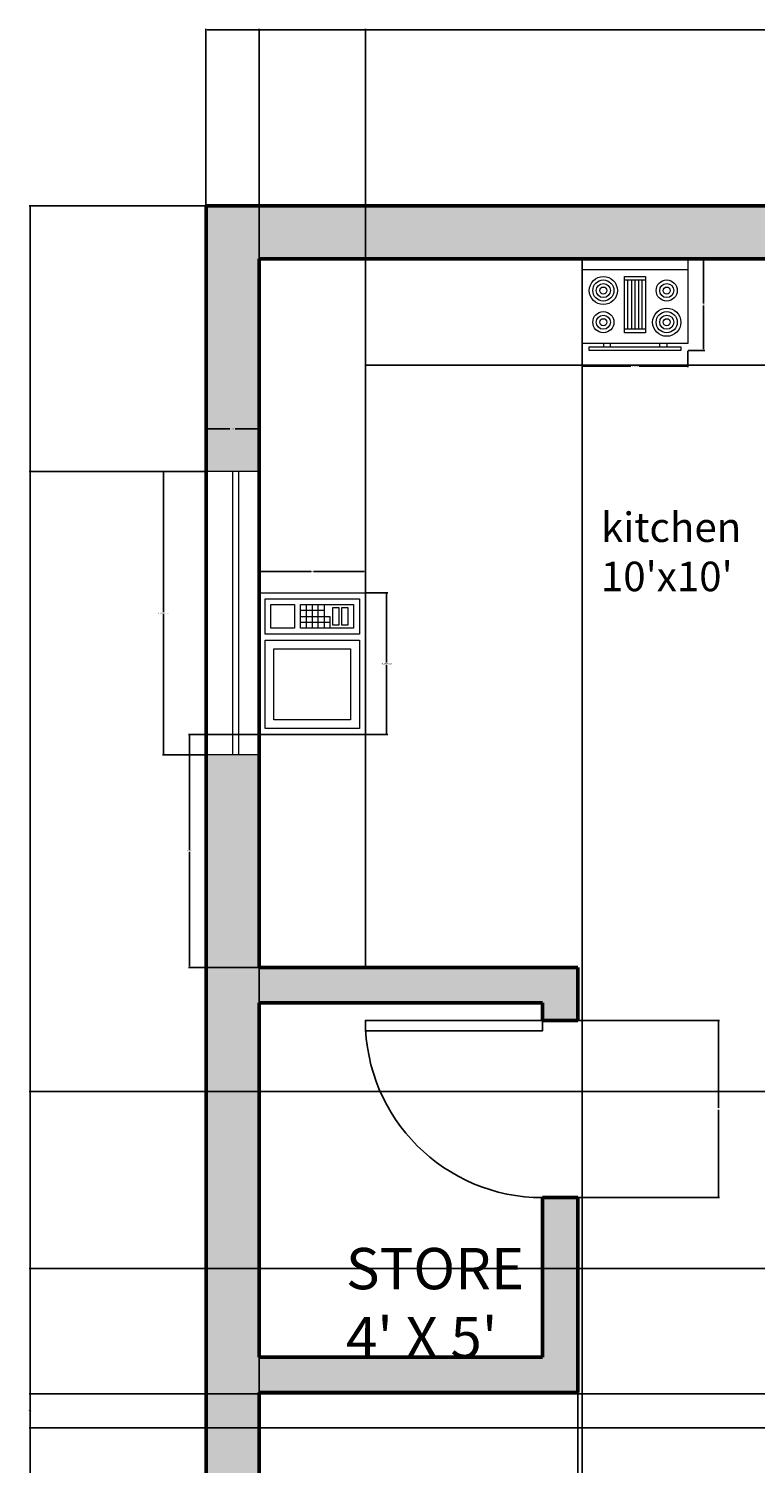
# Model space of a CAD drawing. Units: inches. Extents: x 1489 to 1813, y 1703 to 2293.
# Tile 3 of 4: x 1489 to 1612, y 2050 to 2293. Entities that reach past the tile are written whole.
import ezdxf

# ---------------------------------------------------------------- set-up
doc = ezdxf.new("R2010")
doc.units = ezdxf.units.IN
doc.header["$LTSCALE"] = 0.4
doc.linetypes.add('HIDDEN', pattern=[9.525, 6.35, -3.175])
for name, color, linetype, lineweight in [('A-ANNO-DIMS', 2, 'Continuous', 18), ('A-AREA-IDEN', 7, 'Continuous', 18), ('A-DOOR', 4, 'Continuous', 25), ('A-EQPM', 9, 'Continuous', 18), ('A-FLOR-CASE', 8, 'Continuous', 25), ('A-GLAZ', 4, 'Continuous', 18), ('A-WALL', 7, 'Continuous', 50)]:
    doc.layers.add(name, color=color, linetype=linetype, lineweight=lineweight)
doc.layers.add('A-WALL-PATT', color=18, linetype='HIDDEN', lineweight=13, true_color=0x000000)
doc.styles.get("Standard").update_dxf_attribs({"font": 'arial.ttf'})
doc.dimstyles.get("Standard").update_dxf_attribs({"dimtxt": 0.18, "dimasz": 0.18, "dimexe": 0.18, "dimexo": 0.0625, "dimgap": 0.09, "dimtad": 0, "dimtih": 1, "dimtoh": 1, "dimdec": 4, "dimzin": 0, "dimdsep": 46, "dimtxsty": 'Standard', "dimcen": 0.09, "dimadec": 0, "dimazin": 0, "dimtfac": 1, "dimtdec": 4, "dimtofl": 0, "dimtmove": 0, "dimatfit": 3, "dimfxl": 1, "dimtolj": 1, "dimtzin": 0, "dimarcsym": 0})

# ---------------------------------------------------------------- blocks, each defined once
blk = doc.blocks.new('*U3')
for p, q in [((0, 0), (0, -6)), ((30, 0), (30, -6))]:
    blk.add_line(p, q)
blk.add_lwpolyline([(0, 0), (0, 30), (1.75, 30), (1.75, 0)], close=True)
blk.add_arc((0, 0), 30, 0, 90)
blk = doc.blocks.new('Range-Oven - 30 in top')
for p, q in [((0, -3), (30, -3)), ((12, -6), (18, -6)), ((13, -20), (13, -6)), ((14, -6), (14, -20)), ((15, -20), (15, -6)), ((16, -6), (16, -20)), ((17, -20), (17, -6)), ((18, -20), (12, -20)), ((6, -24), (6, -25)), ((8, -25), (8, -24)), ((22, -25), (22, -24)), ((24, -24), (24, -25))]:
    blk.add_line(p, q)
for points in [[(0, -24), (0, 0), (30, 0), (30, -24)], [(12, -21), (12, -5), (18, -5), (18, -21)], [(2, -26), (2, -25), (28, -25), (28, -26)]]:
    blk.add_lwpolyline(points, close=True)
for centre, radius in [((6, -9), 4), ((6, -9), 3), ((6, -9), 2), ((6, -9), 1), ((24, -9), 3), ((24, -9), 2), ((24, -9), 1), ((6, -18), 3), ((6, -18), 2), ((24, -18), 4), ((24, -18), 3), ((24, -18), 2), ((6, -18), 1), ((24, -18), 1)]:
    blk.add_circle(centre, radius)
blk = doc.blocks.new('Microwave')
for p, q in [((18, 10), (22, 10)), ((19, 7), (19, 11)), ((20, 11), (20, 7)), ((21, 7), (21, 11)), ((22, 9), (18, 9)), ((18, 8), (22, 8)), ((22, 7), (18, 7)), ((20, 6), (18, 6)), ((19, 6), (19, 7)), ((20, 7), (20, 6))]:
    blk.add_line(p, q)
for points in [[(0, 0), (0, 18), (24, 18), (24, 0)], [(1, 1), (1, 17), (16, 17), (16, 1)], [(2.5, 2.5), (2.5, 15.5), (14.5, 15.5), (14.5, 2.5)], [(17, 1), (17, 17), (23, 17), (23, 1)], [(18, 12), (18, 16), (22, 16), (22, 12)], [(18, 2), (18, 11), (22, 11), (22, 2)], [(18.5, 4.5), (18.5, 5.5), (21.5, 5.5), (21.5, 4.5)], [(18.5, 3), (18.5, 4), (21.5, 4), (21.5, 3)]]:
    blk.add_lwpolyline(points, close=True)
blk = doc.blocks.new('WIN-48IN')
for p, q in [((9, 48), (0, 48)), ((4.5, 48), (4.5, 0)), ((5.5, 48), (5.5, 0)), ((9, 0), (0, 0))]:
    blk.add_line(p, q)
blk = doc.blocks.new('*D14')
at = {"layer": 'A-ANNO-DIMS', "color": 0, "lineweight": -2, "ltscale": 0.4, "transparency": 16777216}
for p, q in [((1518.92, 2218.17), (1511.6, 2218.17)), ((1511.78, 2217.99), (1511.78, 2194.35)), ((1511.78, 2170.35), (1511.78, 2193.99)), ((1518.92, 2170.17), (1511.6, 2170.17))]:
    blk.add_line(p, q, dxfattribs=at)
at = {"layer": 'A-ANNO-DIMS', "color": 0, "ltscale": 0.4, "transparency": 16777216}
for points in [[(1511.75, 2217.99), (1511.81, 2217.99), (1511.78, 2218.17)], [(1511.75, 2170.35), (1511.81, 2170.35), (1511.78, 2170.17)]]:
    blk.add_solid(points, dxfattribs=at)
at = {"layer": 'Defpoints', "color": 0, "ltscale": 0.4, "transparency": 16777216}
for p in [(1511.78, 2218.17), (1518.98, 2218.17), (1518.98, 2170.17)]:
    blk.add_point(p, dxfattribs=at)
at = {"layer": 'A-ANNO-DIMS', "color": 0, "ltscale": 0.4, "transparency": 16777216, "insert": (1511.78, 2194.17), "char_height": 0.18, "attachment_point": 5}
blk.add_mtext('\\A1;WINDOW 48 TYP.', dxfattribs=at)
blk = doc.blocks.new('*D15')
at = {"layer": 'A-ANNO-DIMS', "color": 0, "lineweight": -2, "ltscale": 0.4, "transparency": 16777216}
for p, q in [((1518.98, 2218.23), (1518.98, 2225.55)), ((1519.16, 2225.37), (1523.03, 2225.37)), ((1527.8, 2225.37), (1523.94, 2225.37)), ((1527.98, 2218.23), (1527.98, 2225.55))]:
    blk.add_line(p, q, dxfattribs=at)
at = {"layer": 'A-ANNO-DIMS', "color": 0, "ltscale": 0.4, "transparency": 16777216}
for points in [[(1519.16, 2225.4), (1519.16, 2225.34), (1518.98, 2225.37)], [(1527.8, 2225.4), (1527.8, 2225.34), (1527.98, 2225.37)]]:
    blk.add_solid(points, dxfattribs=at)
at = {"layer": 'Defpoints', "color": 0, "ltscale": 0.4, "transparency": 16777216}
for p in [(1527.98, 2225.37), (1518.98, 2218.17), (1527.98, 2218.17)]:
    blk.add_point(p, dxfattribs=at)
at = {"layer": 'A-ANNO-DIMS', "color": 0, "ltscale": 0.4, "transparency": 16777216, "insert": (1523.48, 2225.37), "char_height": 0.18, "attachment_point": 5}
blk.add_mtext('\\A1;9 TYP.', dxfattribs=at)
blk = doc.blocks.new('*D22')
at = {"layer": 'A-ANNO-DIMS', "color": 0, "lineweight": -2, "ltscale": 0.4, "transparency": 16777216}
for p, q in [((1582.71, 2238.6), (1582.71, 2235.8)), ((1600.6, 2238.6), (1600.6, 2235.8)), ((1582.89, 2235.98), (1590.96, 2235.98)), ((1600.42, 2235.98), (1592.35, 2235.98))]:
    blk.add_line(p, q, dxfattribs=at)
at = {"layer": 'A-ANNO-DIMS', "color": 0, "ltscale": 0.4, "transparency": 16777216}
for points in [[(1582.89, 2236.01), (1582.89, 2235.95), (1582.71, 2235.98)], [(1600.42, 2236.01), (1600.42, 2235.95), (1600.6, 2235.98)]]:
    blk.add_solid(points, dxfattribs=at)
at = {"layer": 'Defpoints', "color": 0, "ltscale": 0.4, "transparency": 16777216}
for p in [(1582.71, 2238.67), (1600.6, 2238.67), (1600.6, 2235.98)]:
    blk.add_point(p, dxfattribs=at)
at = {"layer": 'A-ANNO-DIMS', "color": 0, "ltscale": 0.4, "transparency": 16777216, "insert": (1591.66, 2235.98), "char_height": 0.18, "attachment_point": 5}
blk.add_mtext('\\A1;RANGE 18', dxfattribs=at)
blk = doc.blocks.new('*D23')
at = {"layer": 'A-ANNO-DIMS', "color": 0, "lineweight": -2, "ltscale": 0.4, "transparency": 16777216}
for p, q in [((1600.66, 2254.17), (1603.46, 2254.17)), ((1603.28, 2253.99), (1603.28, 2246.6)), ((1603.28, 2238.85), (1603.28, 2246.24)), ((1600.66, 2238.67), (1603.46, 2238.67))]:
    blk.add_line(p, q, dxfattribs=at)
at = {"layer": 'A-ANNO-DIMS', "color": 0, "ltscale": 0.4, "transparency": 16777216}
for points in [[(1603.25, 2253.99), (1603.31, 2253.99), (1603.28, 2254.17)], [(1603.25, 2238.85), (1603.31, 2238.85), (1603.28, 2238.67)]]:
    blk.add_solid(points, dxfattribs=at)
at = {"layer": 'Defpoints', "color": 0, "ltscale": 0.4, "transparency": 16777216}
for p in [(1600.6, 2254.17), (1603.28, 2254.17), (1600.6, 2238.67)]:
    blk.add_point(p, dxfattribs=at)
at = {"layer": 'A-ANNO-DIMS', "color": 0, "ltscale": 0.4, "transparency": 16777216, "insert": (1603.28, 2246.42), "char_height": 0.18, "attachment_point": 5}
blk.add_mtext('\\A1;16', dxfattribs=at)
blk = doc.blocks.new('*D24')
at = {"layer": 'A-ANNO-DIMS', "color": 0, "lineweight": -2, "ltscale": 0.4, "transparency": 16777216}
for p, q in [((1546.05, 2197.6), (1549.76, 2197.6)), ((1549.58, 2197.42), (1549.58, 2185.79)), ((1549.58, 2173.78), (1549.58, 2185.42)), ((1546.05, 2173.6), (1549.76, 2173.6))]:
    blk.add_line(p, q, dxfattribs=at)
at = {"layer": 'A-ANNO-DIMS', "color": 0, "ltscale": 0.4, "transparency": 16777216}
for points in [[(1549.55, 2197.42), (1549.61, 2197.42), (1549.58, 2197.6)], [(1549.55, 2173.78), (1549.61, 2173.78), (1549.58, 2173.6)]]:
    blk.add_solid(points, dxfattribs=at)
at = {"layer": 'Defpoints', "color": 0, "ltscale": 0.4, "transparency": 16777216}
for p in [(1545.98, 2197.6), (1549.58, 2197.6), (1545.98, 2173.6)]:
    blk.add_point(p, dxfattribs=at)
at = {"layer": 'A-ANNO-DIMS', "color": 0, "ltscale": 0.4, "transparency": 16777216, "insert": (1549.58, 2185.6), "char_height": 0.18, "attachment_point": 5}
blk.add_mtext('\\A1;MICROWAVE 24', dxfattribs=at)
blk = doc.blocks.new('*D25')
at = {"layer": 'A-ANNO-DIMS', "color": 0, "lineweight": -2, "ltscale": 0.4, "transparency": 16777216}
for p, q in [((1527.98, 2197.67), (1527.98, 2201.38)), ((1528.16, 2201.2), (1536.77, 2201.2)), ((1545.8, 2201.2), (1537.19, 2201.2)), ((1545.98, 2197.67), (1545.98, 2201.38))]:
    blk.add_line(p, q, dxfattribs=at)
at = {"layer": 'A-ANNO-DIMS', "color": 0, "ltscale": 0.4, "transparency": 16777216}
for points in [[(1528.16, 2201.23), (1528.16, 2201.17), (1527.98, 2201.2)], [(1545.8, 2201.23), (1545.8, 2201.17), (1545.98, 2201.2)]]:
    blk.add_solid(points, dxfattribs=at)
at = {"layer": 'Defpoints', "color": 0, "ltscale": 0.4, "transparency": 16777216}
for p in [(1527.98, 2201.2), (1527.98, 2197.6), (1545.98, 2197.6)]:
    blk.add_point(p, dxfattribs=at)
at = {"layer": 'A-ANNO-DIMS', "color": 0, "ltscale": 0.4, "transparency": 16777216, "insert": (1536.98, 2201.2), "char_height": 0.18, "attachment_point": 5}
blk.add_mtext('\\A1;18', dxfattribs=at)
blk = doc.blocks.new('*D28')
at = {"layer": 'A-ANNO-DIMS', "color": 0, "lineweight": -2, "ltscale": 0.4, "transparency": 16777216}
for p, q in [((1518.98, 2263.23), (1518.98, 2293.15)), ((1519.16, 2292.97), (1650.69, 2292.97)), ((1782.8, 2292.97), (1651.27, 2292.97)), ((1782.98, 2263.23), (1782.98, 2293.15))]:
    blk.add_line(p, q, dxfattribs=at)
at = {"layer": 'A-ANNO-DIMS', "color": 0, "ltscale": 0.4, "transparency": 16777216}
for points in [[(1519.16, 2293), (1519.16, 2292.94), (1518.98, 2292.97)], [(1782.8, 2293), (1782.8, 2292.94), (1782.98, 2292.97)]]:
    blk.add_solid(points, dxfattribs=at)
at = {"layer": 'Defpoints', "color": 0, "ltscale": 0.4, "transparency": 16777216}
for p in [(1782.98, 2292.97), (1518.98, 2263.17), (1782.98, 2263.17)]:
    blk.add_point(p, dxfattribs=at)
at = {"layer": 'A-ANNO-DIMS', "color": 0, "ltscale": 0.4, "transparency": 16777216, "insert": (1650.98, 2292.97), "char_height": 0.18, "attachment_point": 5}
blk.add_mtext('\\A1;264', dxfattribs=at)
blk = doc.blocks.new('*D29')
at = {"layer": 'A-ANNO-DIMS', "color": 0, "lineweight": -2, "ltscale": 0.4, "transparency": 16777216}
for p, q in [((1518.92, 2263.17), (1489, 2263.17)), ((1489.18, 2262.99), (1489.18, 2013.35)), ((1489.18, 1763.35), (1489.18, 2012.99)), ((1602.92, 1763.17), (1489, 1763.17))]:
    blk.add_line(p, q, dxfattribs=at)
at = {"layer": 'A-ANNO-DIMS', "color": 0, "ltscale": 0.4, "transparency": 16777216}
for points in [[(1489.15, 2262.99), (1489.21, 2262.99), (1489.18, 2263.17)], [(1489.15, 1763.35), (1489.21, 1763.35), (1489.18, 1763.17)]]:
    blk.add_solid(points, dxfattribs=at)
at = {"layer": 'Defpoints', "color": 0, "ltscale": 0.4, "transparency": 16777216}
for p in [(1489.18, 2263.17), (1518.98, 2263.17), (1602.98, 1763.17)]:
    blk.add_point(p, dxfattribs=at)
at = {"layer": 'A-ANNO-DIMS', "color": 0, "ltscale": 0.4, "transparency": 16777216, "insert": (1489.18, 2013.17), "char_height": 0.18, "attachment_point": 5}
blk.add_mtext('\\A1;500', dxfattribs=at)
blk = doc.blocks.new('*D39')
at = {"layer": 'A-ANNO-DIMS', "color": 0, "lineweight": -2, "ltscale": 0.4, "transparency": 16777216}
for p, q in [((1518.98, 2263.23), (1518.98, 2293.15)), ((1519.16, 2292.97), (1570.2, 2292.97)), ((1621.8, 2292.97), (1570.76, 2292.97)), ((1621.98, 2263.23), (1621.98, 2293.15))]:
    blk.add_line(p, q, dxfattribs=at)
at = {"layer": 'A-ANNO-DIMS', "color": 0, "ltscale": 0.4, "transparency": 16777216}
for points in [[(1519.16, 2293), (1519.16, 2292.94), (1518.98, 2292.97)], [(1621.8, 2293), (1621.8, 2292.94), (1621.98, 2292.97)]]:
    blk.add_solid(points, dxfattribs=at)
at = {"layer": 'Defpoints', "color": 0, "ltscale": 0.4, "transparency": 16777216}
for p in [(1621.98, 2292.97), (1518.98, 2263.17), (1621.98, 2263.17)]:
    blk.add_point(p, dxfattribs=at)
at = {"layer": 'A-ANNO-DIMS', "color": 0, "ltscale": 0.4, "transparency": 16777216, "insert": (1570.48, 2292.97), "char_height": 0.18, "attachment_point": 5}
blk.add_mtext('\\A1;103', dxfattribs=at)
blk = doc.blocks.new('*D45')
at = {"layer": 'A-ANNO-DIMS', "color": 0, "lineweight": -2, "ltscale": 0.4, "transparency": 16777216}
for p, q in [((1518.92, 2263.17), (1489, 2263.17)), ((1489.18, 2262.99), (1489.18, 2240.85)), ((1489.18, 2218.35), (1489.18, 2240.49)), ((1518.92, 2218.17), (1489, 2218.17))]:
    blk.add_line(p, q, dxfattribs=at)
at = {"layer": 'A-ANNO-DIMS', "color": 0, "ltscale": 0.4, "transparency": 16777216}
for points in [[(1489.15, 2262.99), (1489.21, 2262.99), (1489.18, 2263.17)], [(1489.15, 2218.35), (1489.21, 2218.35), (1489.18, 2218.17)]]:
    blk.add_solid(points, dxfattribs=at)
at = {"layer": 'Defpoints', "color": 0, "ltscale": 0.4, "transparency": 16777216}
for p in [(1489.18, 2263.17), (1518.98, 2263.17), (1518.98, 2218.17)]:
    blk.add_point(p, dxfattribs=at)
at = {"layer": 'A-ANNO-DIMS', "color": 0, "ltscale": 0.4, "transparency": 16777216, "insert": (1489.18, 2240.67), "char_height": 0.18, "attachment_point": 5}
blk.add_mtext('\\A1;45', dxfattribs=at)
blk = doc.blocks.new('*D47')
at = {"layer": 'A-ANNO-DIMS', "color": 0, "lineweight": -2, "ltscale": 0.4, "transparency": 16777216}
for p, q in [((1701.92, 2113.17), (1489, 2113.17)), ((1489.18, 2112.99), (1489.18, 2098.35)), ((1489.18, 2083.35), (1489.18, 2097.99)), ((1701.92, 2083.17), (1489, 2083.17))]:
    blk.add_line(p, q, dxfattribs=at)
at = {"layer": 'A-ANNO-DIMS', "color": 0, "ltscale": 0.4, "transparency": 16777216}
for points in [[(1489.15, 2112.99), (1489.21, 2112.99), (1489.18, 2113.17)], [(1489.15, 2083.35), (1489.21, 2083.35), (1489.18, 2083.17)]]:
    blk.add_solid(points, dxfattribs=at)
at = {"layer": 'Defpoints', "color": 0, "ltscale": 0.4, "transparency": 16777216}
for p in [(1701.98, 2113.17), (1489.18, 2083.17), (1701.98, 2083.17)]:
    blk.add_point(p, dxfattribs=at)
at = {"layer": 'A-ANNO-DIMS', "color": 0, "ltscale": 0.4, "transparency": 16777216, "insert": (1489.18, 2098.17), "char_height": 0.18, "attachment_point": 5}
blk.add_mtext('\\A1;30', dxfattribs=at)
blk = doc.blocks.new('*D48')
at = {"layer": 'A-ANNO-DIMS', "color": 0, "lineweight": -2, "ltscale": 0.4, "transparency": 16777216}
for p, q in [((1576.05, 2125.17), (1605.96, 2125.17)), ((1605.78, 2124.99), (1605.78, 2110.35)), ((1605.78, 2095.35), (1605.78, 2109.99)), ((1576.05, 2095.17), (1605.96, 2095.17))]:
    blk.add_line(p, q, dxfattribs=at)
at = {"layer": 'A-ANNO-DIMS', "color": 0, "ltscale": 0.4, "transparency": 16777216}
for points in [[(1605.75, 2124.99), (1605.81, 2124.99), (1605.78, 2125.17)], [(1605.75, 2095.35), (1605.81, 2095.35), (1605.78, 2095.17)]]:
    blk.add_solid(points, dxfattribs=at)
at = {"layer": 'Defpoints', "color": 0, "ltscale": 0.4, "transparency": 16777216}
for p in [(1575.98, 2125.17), (1575.98, 2095.17), (1605.78, 2095.17)]:
    blk.add_point(p, dxfattribs=at)
at = {"layer": 'A-ANNO-DIMS', "color": 0, "ltscale": 0.4, "transparency": 16777216, "insert": (1605.78, 2110.17), "char_height": 0.18, "attachment_point": 5}
blk.add_mtext('\\A1;30', dxfattribs=at)
blk = doc.blocks.new('*D51')
at = {"layer": 'A-ANNO-DIMS', "color": 0, "lineweight": -2, "ltscale": 0.4, "transparency": 16777216}
for p, q in [((1527.98, 2134.23), (1527.98, 2293.15)), ((1528.16, 2292.97), (1536.77, 2292.97)), ((1545.8, 2292.97), (1537.19, 2292.97)), ((1545.98, 2134.23), (1545.98, 2293.15))]:
    blk.add_line(p, q, dxfattribs=at)
at = {"layer": 'A-ANNO-DIMS', "color": 0, "ltscale": 0.4, "transparency": 16777216}
for points in [[(1528.16, 2293), (1528.16, 2292.94), (1527.98, 2292.97)], [(1545.8, 2293), (1545.8, 2292.94), (1545.98, 2292.97)]]:
    blk.add_solid(points, dxfattribs=at)
at = {"layer": 'Defpoints', "color": 0, "ltscale": 0.4, "transparency": 16777216}
for p in [(1527.98, 2292.97), (1527.98, 2134.17), (1545.98, 2134.17)]:
    blk.add_point(p, dxfattribs=at)
at = {"layer": 'A-ANNO-DIMS', "color": 0, "ltscale": 0.4, "transparency": 16777216, "insert": (1536.98, 2292.97), "char_height": 0.18, "attachment_point": 5}
blk.add_mtext('\\A1;18', dxfattribs=at)
blk = doc.blocks.new('*D52')
at = {"layer": 'A-ANNO-DIMS', "color": 0, "lineweight": -2, "ltscale": 0.4, "transparency": 16777216}
for p, q in [((1527.98, 2254.11), (1527.98, 1705.95)), ((1582.71, 2254.11), (1582.71, 1705.95)), ((1528.16, 1706.13), (1554.95, 1706.13)), ((1582.53, 1706.13), (1555.74, 1706.13))]:
    blk.add_line(p, q, dxfattribs=at)
at = {"layer": 'A-ANNO-DIMS', "color": 0, "ltscale": 0.4, "transparency": 16777216}
for points in [[(1528.16, 1706.16), (1528.16, 1706.1), (1527.98, 1706.13)], [(1582.53, 1706.16), (1582.53, 1706.1), (1582.71, 1706.13)]]:
    blk.add_solid(points, dxfattribs=at)
at = {"layer": 'Defpoints', "color": 0, "ltscale": 0.4, "transparency": 16777216}
for p in [(1527.98, 2254.17), (1582.71, 2254.17), (1582.71, 1706.13)]:
    blk.add_point(p, dxfattribs=at)
at = {"layer": 'A-ANNO-DIMS', "color": 0, "ltscale": 0.4, "transparency": 16777216, "insert": (1555.35, 1706.13), "char_height": 0.18, "attachment_point": 5}
blk.add_mtext('\\A1;54.73', dxfattribs=at)
blk = doc.blocks.new('*D54')
at = {"layer": 'A-ANNO-DIMS', "color": 0, "lineweight": -2, "ltscale": 0.4, "transparency": 16777216}
for p, q in [((1545.92, 2173.6), (1516, 2173.6)), ((1516.18, 2173.42), (1516.18, 2154.07)), ((1516.18, 2134.35), (1516.18, 2153.71)), ((1545.92, 2134.17), (1516, 2134.17))]:
    blk.add_line(p, q, dxfattribs=at)
at = {"layer": 'A-ANNO-DIMS', "color": 0, "ltscale": 0.4, "transparency": 16777216}
for points in [[(1516.15, 2173.42), (1516.21, 2173.42), (1516.18, 2173.6)], [(1516.15, 2134.35), (1516.21, 2134.35), (1516.18, 2134.17)]]:
    blk.add_solid(points, dxfattribs=at)
at = {"layer": 'Defpoints', "color": 0, "ltscale": 0.4, "transparency": 16777216}
for p in [(1516.18, 2173.6), (1545.98, 2173.6), (1545.98, 2134.17)]:
    blk.add_point(p, dxfattribs=at)
at = {"layer": 'A-ANNO-DIMS', "color": 0, "ltscale": 0.4, "transparency": 16777216, "insert": (1516.18, 2153.89), "char_height": 0.18, "attachment_point": 5}
blk.add_mtext('\\A1;39.434', dxfattribs=at)
blk = doc.blocks.new('*D63')
at = {"layer": 'A-ANNO-DIMS', "color": 0, "lineweight": -2, "ltscale": 0.4, "transparency": 16777216}
for p, q in [((1581.98, 2062.11), (1581.98, 1705.95)), ((1695.98, 2056.11), (1695.98, 1705.95)), ((1582.16, 1706.13), (1638.7, 1706.13)), ((1695.8, 1706.13), (1639.26, 1706.13))]:
    blk.add_line(p, q, dxfattribs=at)
at = {"layer": 'A-ANNO-DIMS', "color": 0, "ltscale": 0.4, "transparency": 16777216}
for points in [[(1582.16, 1706.16), (1582.16, 1706.1), (1581.98, 1706.13)], [(1695.8, 1706.16), (1695.8, 1706.1), (1695.98, 1706.13)]]:
    blk.add_solid(points, dxfattribs=at)
at = {"layer": 'Defpoints', "color": 0, "ltscale": 0.4, "transparency": 16777216}
for p in [(1581.98, 2062.17), (1695.98, 2056.17), (1695.98, 1706.13)]:
    blk.add_point(p, dxfattribs=at)
at = {"layer": 'A-ANNO-DIMS', "color": 0, "ltscale": 0.4, "transparency": 16777216, "insert": (1638.98, 1706.13), "char_height": 0.18, "attachment_point": 5}
blk.add_mtext('\\A1;114', dxfattribs=at)
blk = doc.blocks.new('*D65')
at = {"layer": 'A-ANNO-DIMS', "color": 0, "lineweight": -2, "ltscale": 0.4, "transparency": 16777216}
for p, q in [((1767.83, 2061.91), (1489, 2061.91)), ((1489.18, 2061.73), (1489.18, 2059.22)), ((1489.18, 2056.35), (1489.18, 2058.86)), ((1773.92, 2056.17), (1489, 2056.17))]:
    blk.add_line(p, q, dxfattribs=at)
at = {"layer": 'A-ANNO-DIMS', "color": 0, "ltscale": 0.4, "transparency": 16777216}
for points in [[(1489.15, 2061.73), (1489.21, 2061.73), (1489.18, 2061.91)], [(1489.15, 2056.35), (1489.21, 2056.35), (1489.18, 2056.17)]]:
    blk.add_solid(points, dxfattribs=at)
at = {"layer": 'Defpoints', "color": 0, "ltscale": 0.4, "transparency": 16777216}
for p in [(1767.89, 2061.91), (1489.18, 2056.17), (1773.98, 2056.17)]:
    blk.add_point(p, dxfattribs=at)
at = {"layer": 'A-ANNO-DIMS', "color": 0, "ltscale": 0.4, "transparency": 16777216, "insert": (1489.18, 2059.04), "char_height": 0.18, "attachment_point": 5}
blk.add_mtext('\\A1;5.74', dxfattribs=at)

msp = doc.modelspace()

# ---------------------------------------------------------------- hatches: boundary and pattern name
at = {"layer": 'A-WALL-PATT', "ltscale": 0.4}
h = msp.add_hatch(dxfattribs=at)
h.set_pattern_fill('HONEY', color=256, scale=0.1)
h.paths.add_polyline_path([(1621.9839, 2263.1709), (1518.9839, 2263.1709), (1518.9839, 2218.1709), (1527.9839, 2218.1709), (1527.9839, 2254.1709), (1621.9839, 2254.1709)])
h = msp.add_hatch(dxfattribs=at)
h.set_pattern_fill('HONEY', color=256, scale=0.1)
h.paths.add_polyline_path([(1527.9839, 2128.1709), (1575.9839, 2128.1709), (1575.9839, 2125.1709), (1581.9839, 2125.1709), (1581.9839, 2134.1709), (1527.9839, 2134.1709), (1527.9839, 2170.1709), (1518.9839, 2170.1709), (1518.9839, 2020.1709), (1527.9839, 2020.1709), (1527.9839, 2062.1709), (1581.9839, 2062.1709), (1581.9839, 2095.1709), (1575.9839, 2095.1709), (1575.9839, 2068.1709), (1527.9839, 2068.1709)])
h.paths.add_polyline_path([(1527.9839, 1924.1709), (1608.9839, 1924.1709), (1608.9839, 1930.1709), (1527.9839, 1930.1709), (1527.9839, 1972.1709), (1518.9839, 1972.1709), (1518.9839, 1882.1709), (1527.9839, 1882.1709)])
h.paths.add_polyline_path([(1527.9839, 1834.1709), (1518.9839, 1834.1709), (1518.9839, 1783.1709), (1614.9839, 1783.1709), (1614.9839, 1789.1709), (1614.9839, 1792.1709), (1527.9839, 1792.1709)])
h.paths.add_polyline_path([(1782.9839, 1867.1709), (1773.9839, 1867.1709), (1773.9839, 1846.1709), (1647.9839, 1846.1709), (1647.9839, 1840.1709), (1773.9839, 1840.1709), (1773.9839, 1792.1709), (1650.9839, 1792.1709), (1650.9839, 1783.1709), (1782.9839, 1783.1709)])
h.paths.add_polyline_path([(1540.5005, 2064.0337), (1577.6874, 2064.0337), (1577.6874, 2090.1253), (1540.5005, 2090.1253)], flags=24)

# ---------------------------------------------------------------- linework, layer by layer
at = {"layer": 'A-FLOR-CASE'}
for p, q in [((1647.9839, 2236.1709), (1545.9839, 2236.1709)), ((1545.9839, 2236.1709), (1545.9839, 2134.1709))]:
    msp.add_line(p, q, dxfattribs=at)
at = {"layer": 'A-WALL'}
for p, q in [((1782.9839, 2263.1709), (1518.9839, 2263.1709)), ((1518.9839, 2263.1709), (1518.9839, 1783.1709)), ((1527.9839, 2254.1709), (1527.9839, 2134.1709)), ((1647.9839, 2254.1709), (1527.9839, 2254.1709)), ((1581.9839, 2134.1709), (1527.9839, 2134.1709)), ((1581.9839, 2134.1709), (1581.9839, 2125.1709)), ((1575.9839, 2128.1709), (1527.9839, 2128.1709)), ((1527.9839, 2128.1709), (1527.9839, 2068.1709)), ((1575.9839, 2128.1709), (1575.9839, 2125.1709)), ((1575.9839, 2125.1709), (1581.9839, 2125.1709)), ((1575.9839, 2095.1709), (1581.9839, 2095.1709)), ((1575.9839, 2095.1709), (1575.9839, 2068.1709)), ((1581.9839, 2095.1709), (1581.9839, 2062.1709)), ((1575.9839, 2068.1709), (1527.9839, 2068.1709)), ((1581.9839, 2062.1709), (1527.9839, 2062.1709)), ((1527.9839, 2062.1709), (1527.9839, 1930.1709))]:
    msp.add_line(p, q, dxfattribs=at)

# ---------------------------------------------------------------- block references
at = {"layer": 'A-DOOR', "xscale": -1, "rotation": 90}
msp.add_blockref('*U3', (1575.9839, 2125.1709), dxfattribs=at)
at = {"layer": 'A-EQPM', "xscale": 0.5962846747429749, "yscale": 0.5962846747429749, "zscale": 0.5962846747429749}
msp.add_blockref('Range-Oven - 30 in top', (1582.7115, 2254.1709), dxfattribs=at)
at = {"layer": 'A-EQPM', "rotation": 90}
msp.add_blockref('Microwave', (1545.9839, 2173.6048), dxfattribs=at)
at = {"layer": 'A-GLAZ'}
msp.add_blockref('WIN-48IN', (1518.984, 2170.171), dxfattribs=at)

# ---------------------------------------------------------------- texts
at = {"layer": 'A-AREA-IDEN', "attachment_point": 1}
for s, width, insert, char_height in [("kitchen\\P10'x10'", 8.380916, (1585.8776, 2211.2161), 5), ("STORE\\P4' X 5'", 29.471135, (1542.6898, 2086.6468), 7)]:
    msp.add_mtext_dynamic_manual_height_columns(s, width=width, gutter_width=12.5, heights=[0], dxfattribs=dict(at, insert=insert, char_height=char_height))

# ---------------------------------------------------------------- dimensions: what is measured, and where the dimension line sits
at = {"layer": 'A-ANNO-DIMS', "ltscale": 0.4}
for base, p1, p2, override, picture, middle in [((1782.9839, 2292.9709), (1518.9839, 2263.1709), (1782.9839, 2263.1709), {"dimdec": 0, "dimlfac": 1, "dimrnd": 0, "dimzin": 0, "dimdsep": 46, "dimlunit": 2}, '*D28', (1650.9839, 2292.9709)), ((1621.9839, 2292.9709), (1518.9839, 2263.1709), (1621.9839, 2263.1709), {"dimdec": 0, "dimlfac": 1, "dimrnd": 0, "dimzin": 0, "dimdsep": 46, "dimlunit": 2}, '*D39', (1570.4839, 2292.9709)), ((1527.9839, 2292.9709), (1545.9839, 2134.1709), (1527.9839, 2134.1709), {"dimdec": 0, "dimlfac": 1, "dimrnd": 0, "dimzin": 0, "dimdsep": 46, "dimlunit": 2}, '*D51', (1536.9839, 2292.9709)), ((1582.7115, 1706.1265), (1527.9839, 2254.1709), (1582.7115, 2254.1709), {"dimdec": 2, "dimlfac": 1, "dimrnd": 0, "dimzin": 0, "dimdsep": 46, "dimlunit": 2}, '*D52', (1555.3477, 1706.1265)), ((1695.9839, 1706.1265), (1581.9839, 2062.1709), (1695.9839, 2056.1709), {"dimdec": 0, "dimlfac": 1, "dimrnd": 0, "dimzin": 0, "dimdsep": 46, "dimlunit": 2}, '*D63', (1638.9839, 1706.1265))]:
    dim = msp.add_linear_dim(base=base, p1=p1, p2=p2, dimstyle='Standard', override=override, dxfattribs=at)
    dim.commit()
    dim.dimension.update_dxf_attribs({"geometry": picture, "text_midpoint": middle})
for base, p1, p2, angle, override, picture, middle in [((1489.1839, 2263.1709), (1602.9839, 1763.1709), (1518.9839, 2263.1709), 90, {"dimdec": 0, "dimlfac": 1, "dimrnd": 0, "dimzin": 0, "dimdsep": 46, "dimlunit": 2}, '*D29', (1489.1839, 2013.1709)), ((1489.1839, 2263.1709), (1518.9839, 2218.1709), (1518.9839, 2263.1709), 90, {"dimdec": 0, "dimlfac": 1, "dimrnd": 0, "dimzin": 0, "dimdsep": 46, "dimlunit": 2}, '*D45', (1489.1839, 2240.6709)), ((1603.2834, 2254.1709), (1600.6001, 2238.6675), (1600.6001, 2254.1709), 90, {"dimdec": 0, "dimlfac": 1, "dimrnd": 0, "dimzin": 0, "dimdsep": 46, "dimlunit": 2}, '*D23', (1603.2834, 2246.4192)), ((1527.9839, 2201.2048), (1545.9839, 2197.6048), (1527.9839, 2197.6048), 180, {"dimdec": 0, "dimlfac": 1, "dimrnd": 0, "dimzin": 0, "dimdsep": 46, "dimlunit": 2}, '*D25', (1536.9839, 2201.2048)), ((1516.1839, 2173.6048), (1545.9839, 2134.1709), (1545.9839, 2173.6048), 90, {"dimdec": 3, "dimlfac": 1, "dimrnd": 0, "dimzin": 0, "dimdsep": 46, "dimlunit": 2}, '*D54', (1516.1839, 2153.8879)), ((1605.7839, 2095.1709), (1575.9839, 2125.1709), (1575.9839, 2095.1709), 270, {"dimdec": 0, "dimlfac": 1, "dimrnd": 0, "dimzin": 0, "dimdsep": 46, "dimlunit": 2}, '*D48', (1605.7839, 2110.1709)), ((1489.1839, 2083.1709), (1701.9839, 2113.1709), (1701.9839, 2083.1709), 90, {"dimdec": 0, "dimlfac": 1, "dimrnd": 0, "dimzin": 0, "dimdsep": 46, "dimlunit": 2}, '*D47', (1489.1839, 2098.1709)), ((1489.1839, 2056.1709), (1767.8924, 2061.9104), (1773.9839, 2056.1709), 90, {"dimdec": 2, "dimlfac": 1, "dimrnd": 0, "dimzin": 0, "dimdsep": 46, "dimlunit": 2}, '*D65', (1489.1839, 2059.0406))]:
    dim = msp.add_linear_dim(base=base, p1=p1, p2=p2, angle=angle, dimstyle='Standard', override=override, dxfattribs=at)
    dim.commit()
    dim.dimension.update_dxf_attribs({"geometry": picture, "text_midpoint": middle})
for base, p1, p2, text, picture, middle in [((1600.6001, 2235.9842), (1582.7115, 2238.6675), (1600.6001, 2238.6675), 'RANGE <>', '*D22', (1591.6558, 2235.9842)), ((1527.9839, 2225.3709), (1518.9839, 2218.1709), (1527.9839, 2218.1709), '<> TYP.', '*D15', (1523.4839, 2225.3709))]:
    dim = msp.add_linear_dim(base=base, p1=p1, p2=p2, text=text, dimstyle='Standard', override={"dimdec": 0, "dimlfac": 1, "dimrnd": 0, "dimzin": 0, "dimdsep": 46, "dimlunit": 2}, dxfattribs=at)
    dim.commit()
    dim.dimension.update_dxf_attribs({"geometry": picture, "text_midpoint": middle})
for base, p1, p2, text, picture, middle in [((1511.7839, 2218.1709), (1518.9839, 2170.1709), (1518.9839, 2218.1709), 'WINDOW <> TYP.', '*D14', (1511.7839, 2194.1709)), ((1549.5839, 2197.6048), (1545.9839, 2173.6048), (1545.9839, 2197.6048), 'MICROWAVE <>', '*D24', (1549.5839, 2185.6048))]:
    dim = msp.add_linear_dim(base=base, p1=p1, p2=p2, angle=90, text=text, dimstyle='Standard', override={"dimdec": 0, "dimlfac": 1, "dimrnd": 0, "dimzin": 0, "dimdsep": 46, "dimlunit": 2}, dxfattribs=at)
    dim.commit()
    dim.dimension.update_dxf_attribs({"geometry": picture, "text_midpoint": middle})

doc.saveas('drawing.dxf')
